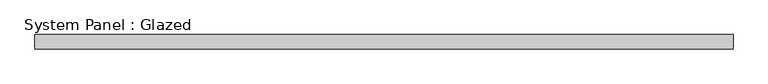
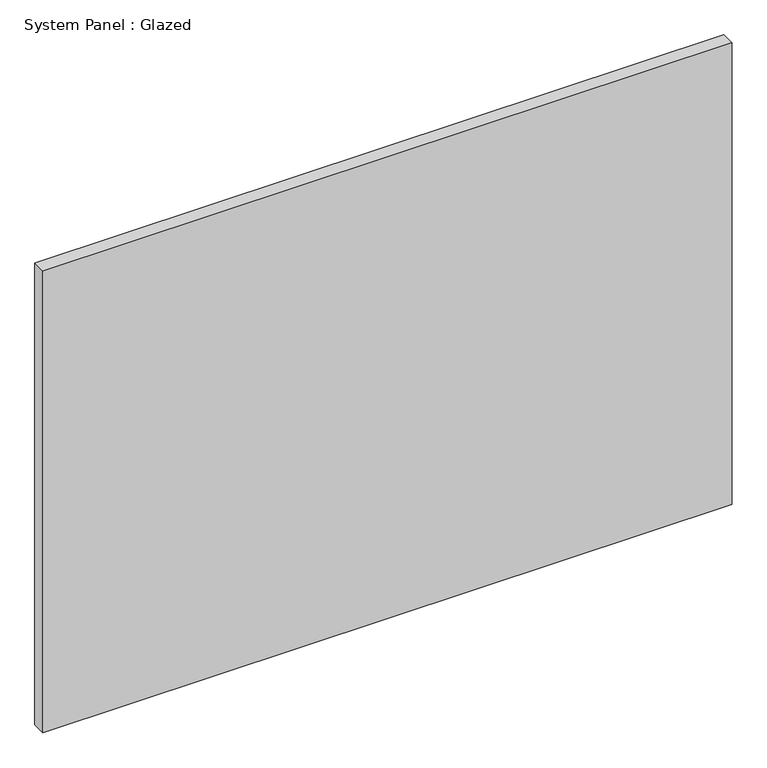
"""IFC4 building model written with IfcOpenShell, lengths in millimetres: plate geometry, System Panel : Glazed."""

from ifc_helpers import new_model, si_unit, origin, origin_with_axes, place, context, project, spatial, polyline, outline, extrude, source, transform, mapped, element, save


def system_panel_glazed_36a05233(model_context):
    return source(origin(), model_context, "Body", "SweptSolid", [
        extrude(outline(polyline([(628.65, 19.05), (-628.65, 19.05), (-628.65, 44.45), (628.65, 44.45), (628.65, 19.05)])), origin_with_axes(), (0.0, 0.0, 1.0), 890.928642),
    ])


if __name__ == "__main__":
    model = new_model("IFC4")
    model_context = context("Model", 3, world=origin())
    ifc_project = project(units=[si_unit("LENGTHUNIT", "METRE", prefix="MILLI")], contexts=[model_context])
    site = spatial("IfcSite", under=ifc_project)
    building = spatial("IfcBuilding", under=site)
    placement = place(None, origin())
    system_panel_glazed_shape = system_panel_glazed_36a05233(model_context)
    element("IfcPlate", 1, ObjectType="System Panel : Glazed", at=placement, inside=building, context=model_context, shape_type="MappedRepresentation", body=[
        mapped(system_panel_glazed_shape, transform((0.0, 0.0, 0.0), x_axis=(1.0, 0.0, 0.0), y_axis=(0.0, 1.0, 0.0), z_axis=(0.0, 0.0, 1.0))),
    ])
    save(model, "model.ifc")

# Revit data of these elements
# Type "System Panel : Glazed"
#   Construction Type Id = "GSP4R"
#   Analytic Construction = "1/8 in Pilkington single glazing"
#   Visual Light Transmittance = 0.9
#   Solar Heat Gain Coefficient = 0.86
#   Heat Transfer Coefficient (U) = 1.18115 BTU/(h·ft²·°F)
#   Define Thermal Properties by = 1
# Element 1 (IfcPlate, "System Panel : Glazed")
#   Materials on its faces: "Glass"
# Materials
#   "Glass": class "Glass", colour RGB 0 128 192, transparency 0.75, Description = "Soda Lime Glass", Cost = 0
